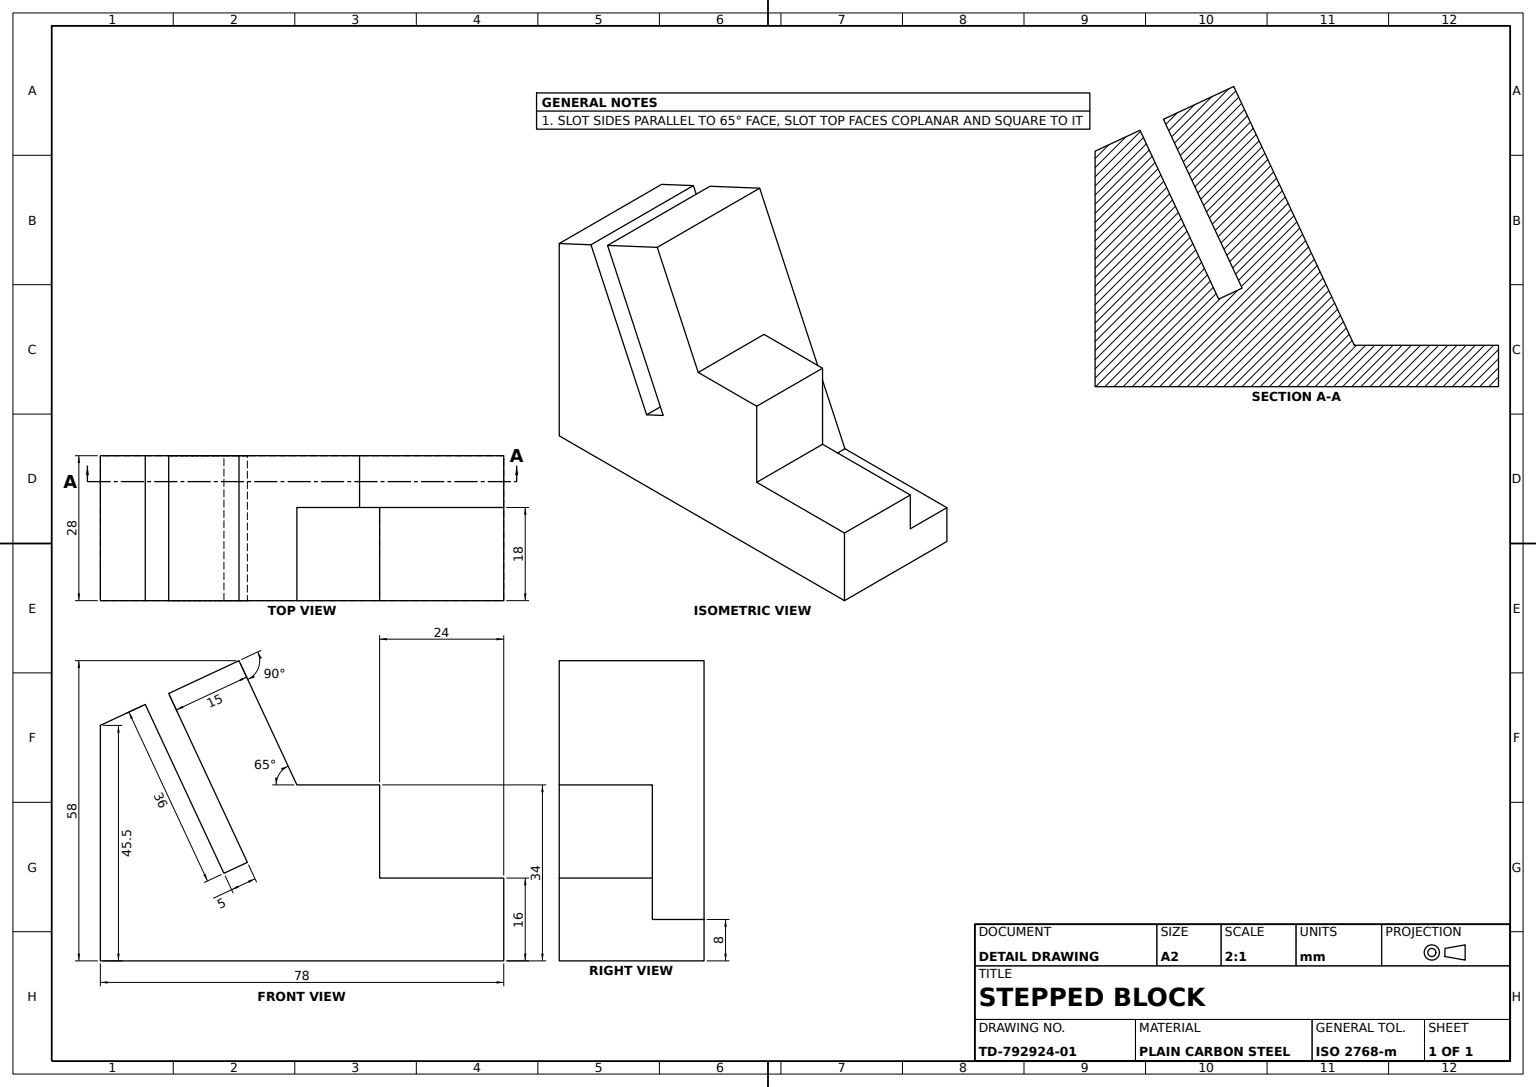
SolidWorks part; units mm, degrees
material "Plain Carbon Steel"
ref_plane "Front Plane" through (0, 0, 0) normal (0, 0, 1) x (1, 0, 0)
ref_plane "Top Plane" through (0, 0, 0) normal (0, 1, 0) x (1, 0, 0)
ref_plane "Right Plane" through (0, 0, 0) normal (1, 0, 0) x (0, 0, -1)
sketch "Base Plate Sketch" plane through (0, 0, 0) normal (0, 1, 0) x (1, 0, 0)
  line L1 (-39, 14) -> (39, 14)
  line L2 (-39, 14) -> (-39, -14)
  line L3 (-39, -14) -> (39, -14)
  line L4 (39, 14) -> (39, -14)
  line L5 (-39, 14) -> (39, -14) construction
  line L6 (-39, -14) -> (39, 14) construction
  point P0 (0, 0)
  dimension "D1" = 28
  dimension "D2" = 78
extrude "Base Plate 78x28x8" add sketch "Base Plate Sketch" along normal blind 8
sketch "V-Notch Upright Sketch" plane through (0, 0, 14) normal (0, 0, 1) x (1, 0, 0)
  line L0 (-11.124, 8) -> (12.1914, 58)
  line L1 (-39, 8) -> (39, 8) construction
  line L2 (12.1914, 58) -> (25.786, 51.6607)
  line L3 (25.786, 51.6607) -> (10.5717, 19.0336)
  line L4 (10.5717, 19.0336) -> (15.1033, 16.9206)
  line L5 (15.1033, 16.9206) -> (30.3175, 49.5476)
  line L6 (30.3175, 49.5476) -> (39, 45.4989)
  line L7 (39, 45.4989) -> (39, 8)
  line L8 (-11.124, 8) -> (39, 8)
  dimension "D1" = 65
  dimension "D2" = 36
  dimension "D3" = 29.58
  dimension "D4" = 58
  dimension "D5" = 5
  dimension "D6" = 15
  dimension "D7" = 0
sketch "Step Block Sketch" plane through (0, 0, -14) normal (0, 0, -1) x (-1, 0, 0)
  line L0 (39, 8) -> (39, 16)
  line L1 (39, 16) -> (15, 16)
  line L2 (15, 16) -> (15, 34)
  line L3 (15, 34) -> (-1, 34)
  line L4 (-1, 34) -> (-1, 8)
  line L5 (-39, 8) -> (39, 8) construction
  line L6 (-1, 8) -> (39, 8)
  line L7 (-39, 0) -> (39, 0) construction
  dimension "D1" = 8
  dimension "D2" = 24
  dimension "D3" = 16
  dimension "D4" = 34
  dimension "D5" = 16
  dimension "D6" = 18
extrude "Step Block" add sketch "Step Block Sketch" against normal blind 18
extrude "V-Notch Upright" add sketch "V-Notch Upright Sketch" against normal up to surface (28 mm away) contours L8 L7 L6 L5 L4 L3 L2 L0 up to face at (-3.5, 14.5, -14)
